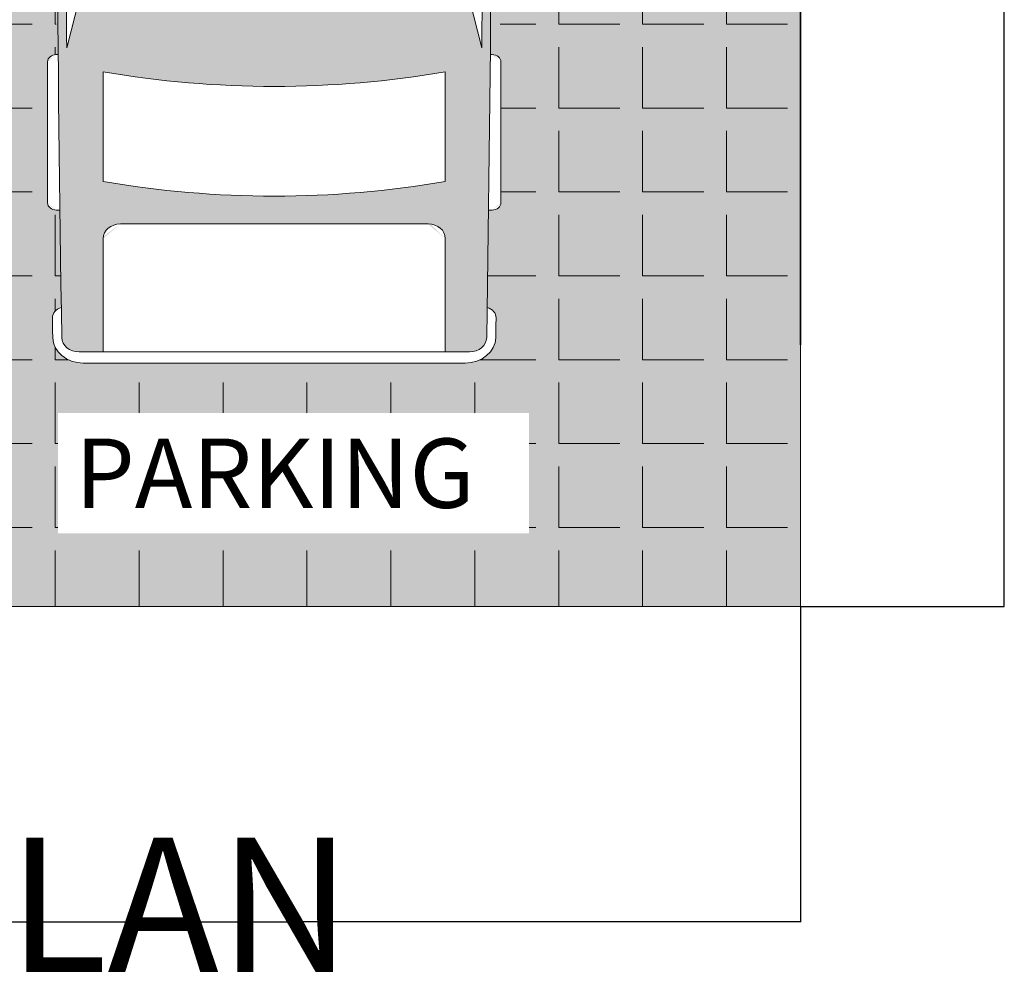
# Model space of a CAD drawing. Units: millimetres. Extents: x 1166 to 16630, y -7192 to 2820.
# Tile 4 of 8: x 5842 to 8218, y -7192 to -4887. Entities that reach past the tile are written whole.
import ezdxf

# ---------------------------------------------------------------- set-up
doc = ezdxf.new("R2010")
doc.units = ezdxf.units.MM
for name, color, linetype, lineweight in [('A-ANNO-DIMS', 2, 'Continuous', 18), ('A-ANNO-TEXT', 7, 'Continuous', 35), ('A-AREA-IDEN', 7, 'Continuous', 18), ('A-FLOR-PATT', 8, 'Continuous', 13), ('A-WALL', 7, 'Continuous', 35), ('C-PKNG-VEHI', 8, 'Continuous', 18), ('C-SITE-PAVE', 7, 'Continuous', 18)]:
    doc.layers.add(name, color=color, linetype=linetype, lineweight=lineweight)
doc.layers.add('A-FLOR-FNSH-PATT', color=254, linetype='Continuous', lineweight=13, true_color=0xfeeab9)
doc.layers.add('C-PKNG-VEHI-PATT', color=18, linetype='Continuous', lineweight=13, true_color=0x000000)
doc.styles.get("Standard").update_dxf_attribs({"font": 'arial.ttf'})
doc.dimstyles.get("Standard").update_dxf_attribs({"dimtxt": 0.18, "dimasz": 0.18, "dimexe": 0.18, "dimexo": 0.0625, "dimgap": 0.09, "dimtad": 0, "dimtih": 1, "dimtoh": 1, "dimdec": 4, "dimzin": 0, "dimdsep": 46, "dimtxsty": 'Standard', "dimcen": 0.09, "dimadec": 0, "dimazin": 0, "dimtfac": 1, "dimtdec": 4, "dimtofl": 0, "dimtmove": 0, "dimatfit": 3, "dimfxl": 1, "dimtolj": 1, "dimtzin": 0, "dimarcsym": 0})

# ---------------------------------------------------------------- blocks, each defined once
blk = doc.blocks.new('*U6')
for p, q in [((46.55368679439944, 38.88847654282876), (22.35054758993934, 38.88847654282876)), ((136.6978032355602, 38.88847654282876), (160.90094244002, 38.88847654282867)), ((21.10406751471477, 37.40863046792069), (21.10406751471477, 36.83230215753705)), ((47.80016686962392, 37.39011648242055), (47.80016686962392, 37.40863046792069)), ((135.4513231603356, 37.07354110333037), (135.4513231603356, 37.40863046792069)), ((162.1474225152445, 37.40863046792049), (162.1474225152445, 36.77402019194128)), ((87.98532186932616, 31.87120872459877), (74.75900729854769, 35.92175679182955)), ((134.313356548143, 35.6043097713567), (119.2882629232503, 31.77757799177584)), ((186.4728846989705, -33.49860931502491), (186.4728846989718, 33.49860931502465)), ((188.3990091454065, -32.75868627757393), (188.3990091454077, 32.75868627757058)), ((70.0302824853563, 31.53613089391356), (86.40615155322342, 29.35124891408057)), ((138.4228833961707, 29.35124891408074), (157.2465674415997, 29.35124891408074)), ((186.4728846989718, 29.35124891408083), (167.0083537481071, 29.35124891408083)), ((164.515393597658, 26.39155676426461), (164.5153935976578, -26.39155676426503)), ((32.26591480791686, 11.62530558863241), (36.12873726252356, 17.16961494239206)), ((36.12873726252356, 17.16961494239206), (50.93891189819171, 17.16961494239206)), ((32.12291633764599, 9.505833383620029), (32.12291633764599, 11.15369945057711)), ((58.9167604809788, -10.77488335095668), (58.9167604809788, 10.77488335095617)), ((66.55009204259746, -10.5288681329018), (66.55009204259746, 10.52886813290129)), ((186.4728846989718, -10.5288681329018), (186.4728846989718, 10.52886813290129)), ((29.77279020470884, 9.505833383620029), (51.68362801571248, 9.505833383620029)), ((82.73706193978568, 8.496039918672748), (82.73706193978568, -8.49603991867258)), ((3.266462181856987, 6.128290093440767), (0.1022408397004821, 0.4060708604429806)), ((-4.43e-14, -2.558e-13), (51.68362801571248, -2.558e-13)), ((0.1022408397004821, -0.4060708604432933), (3.266462181856987, -6.128290093441194)), ((29.77279020470884, -9.50583338362054), (51.68362801571248, -9.50583338362054)), ((32.12291633764599, -9.50583338362054), (32.12291633764599, -11.15369945057762)), ((32.26591480791686, -11.62530558863292), (36.12873726252356, -17.16961494239257)), ((36.12873726252356, -17.16961494239257), (50.93891189819171, -17.16961494239257)), ((86.40615155322318, -29.35124891408145), (70.03028248535594, -31.53613089391442)), ((157.2465674415997, -29.35124891408117), (138.4228833961707, -29.35124891408126)), ((167.008353748107, -29.35124891408126), (186.4728846989707, -29.35124891408108)), ((87.98532186932607, -31.87120872459903), (74.7590072985476, -35.92175679182964)), ((134.3133565481428, -35.60430977135721), (119.2882629232503, -31.77757799177618)), ((21.10406751471477, -37.4086304679212), (21.10406751471477, -36.83230215753756)), ((135.4513231603355, -37.07354110333088), (135.4513231603355, -37.4086304679212)), ((162.1474225152445, -37.408630467921), (162.1474225152445, -36.77402019194179)), ((47.80016686962392, -37.39011648242107), (47.80016686962392, -37.4086304679212)), ((46.55368679439944, -38.88847654282927), (22.35054758993934, -38.88847654282927)), ((136.6978032355602, -38.88847654282927), (160.9009424400199, -38.88847654282918))]:
    blk.add_line(p, q)
for centre, major_axis, ratio, start_param, end_param in [((22.35054758993934, 37.40863046792072), (2.08e-14, -1.479846074908118), 0.842303869543976, 3.141592653589776, 4.712388980384677), ((46.55368679439944, 37.40863046792072), (2.2e-14, 1.479846074908118), 0.8423038695439758, -1.570796326794884, 1.73e-14), ((136.6978032355602, 37.40863046792072), (2.357e-13, -1.479846074908118), 0.842303869543976, 3.141592653589603, 4.712388980384554), ((160.90094244002, 37.40863046792052), (5.59e-14, 1.479846074908118), 0.842303869543976, -1.570796326794865, 4.44e-14), ((41.19115208863305, -490.8631038926156), (1.294e-13, 528.2339998381949), 0.8423038695439741, 0.0028100083536837, 0.0755983031096952), ((64.48199294511879, -10555.61767587835), (1.907644e-10, 10593.02630634627), 0.842303869543847, -0.0133969486112073, 0.0027970409639888), ((180.6280394947615, 35.8381667808375), (7.4e-14, 2.219769112362114), 0.8423038695439693, -0.0130174256259048, 1.249894140392862), ((64.48199294754608, -10556.35759891604), (1.349839377e-06, 10595.3130398087), 0.8423038681351469, -0.0133969484821159, -0.0130174254969711), ((183.9799245485216, 32.75868627756583), (8.56e-14, -5.246425615115243), 0.8423038695439737, 1.570796326795794, 3.128195704978164), ((266.0300214172791, -27.52442688366631), (1.966072e-10, 313.3077612809058), 0.8423038695435284, 1.367075990158062, 1.391760499156098), ((64.4819929449925, -10555.61767590795), (1.9177683e-09, -10591.54646030096), 0.8423038695482963, 3.133765086725325, 3.140440689641252), ((183.9799245485226, 33.49860931502124), (3e-16, -2.959692149816168), 0.8423038695439952, 1.570796326796048, 3.128195704978389), ((135.2911776514449, 5.387441675478555), (2.2715e-12, 81.77258453065997), 0.8423038695439563, 1.245306111696802, 1.507880129813836), ((95.78879860270445, -3666.353346297651), (1.949864e-10, -3698.236159209632), 0.8423038695446962, 3.134048706297306, 3.14409775411291), ((37.47375371777758, -593.9621830607928), (6.21e-14, -623.32820996736), 0.8423038695439826, 3.09604606856106, 3.200911180495224), ((149.595361812917, 2.799442537139299), (8.561e-13, -79.57966406425402), 0.842303869543983, 4.372215489277867, 4.640744122441986), ((17.08207736189386, -1.421e-13), (6.87e-14, 147.0179238898305), 0.8423038695439764, 4.511394369635731, 4.913383591133647), ((35.90576140732288, -1.421e-13), (6.87e-14, 147.0179238898305), 0.8423038695439764, 4.511394369635731, 4.913383591133647), ((167.0083537481071, 26.39155676426464), (1.394e-13, 2.959692149816236), 0.842303869543976, 5.55e-14, 1.57079632679492), ((259.1750197310735, -27.52442688366614), (1.506617e-10, -305.3028914627677), 0.8423038695443789, 4.528606069860317, 4.561837674556238), ((134.4003789125686, 5.387441675477674), (4.276e-13, -89.7774543484738), 0.84230386954398, 4.44948196380473, 4.652344057257214), ((-204.4946649195746, 52.39684969293512), (4.12053e-11, -250.9602162198571), 0.8423038695441164, 1.385369446298923, 1.434372047871027), ((13.03653510440275, 17.00972444508943), (1.2303e-12, 27.41599049210566), 0.8423038695439277, 4.435146050259648, 4.718221029521873), ((14.20086229321332, 17.00972444508943), (1.2303e-12, 27.41599049210566), 0.8423038695439277, 4.435146050259648, 4.718221029521873), ((50.7902773840875, 13.33772416300607), (6.340077547122382, -0.356608581037027), 0.6038335755719145, -1.39555193967809, 1.581314658479915), ((32.74615637525823, 11.15369945057713), (1.313e-13, 0.7399230374541176), 0.8423038695439091, 0.8797135699495516, 1.570796326795045), ((29.77279020470884, -46.66302566589627), (5.12e-14, 56.16885904951626), 0.842303869543976, 7e-16, 0.5903187773915901), ((0.6232400376122422, -1.421e-13), (1e-16, -0.7399230374541245), 0.842303869543842, 4.131459131953847, 5.293318828815531), ((29.77279020470884, 46.66302566589578), (4.004e-13, 56.16885904951626), 0.8423038695439734, 2.55127387619821, 3.141592653589801), ((-204.4946649195746, -52.39684969293552), (4.02945e-11, 250.9602162198562), 0.8423038695441192, -1.43437204787103, -1.385369446298926), ((13.03653510440275, -17.00972444508983), (1.2568e-12, -27.41599049210552), 0.8423038695439318, 1.564964277657711, 1.848039256919935), ((14.20086229321332, -17.00972444508983), (1.2568e-12, -27.41599049210552), 0.8423038695439318, 1.564964277657711, 1.848039256919935), ((149.5953618129329, -2.799442537137565), (4.0897e-12, -79.57966406427697), 0.8423038695439419, -1.499151468852248, -1.230622835688196), ((32.74615637525823, -11.1536994505777), (1.3e-13, -0.7399230374541176), 0.8423038695439093, 4.712388980384541, 5.403471737230034), ((134.4003789125684, -5.387441675478584), (4.2949e-12, -89.77745434847827), 0.8423038695439354, -1.510751403667474, -1.307889310215002), ((135.2911776514465, -5.387441675480715), (3.2038e-12, -81.77258453066244), 0.8423038695439492, -1.50788012981387, -1.245306111696839), ((259.1750197310694, 27.52442688365929), (1.08535e-11, 305.3028914629043), 0.8423038695439974, 1.721347632622872, 1.754579237318777), ((167.008353748107, -26.39155676426503), (1.02e-14, -2.959692149816192), 0.8423038695439885, 4.712388980384686, 6.283185307179581), ((266.0300214172791, 27.52442688366566), (8.75241e-11, 313.3077612806533), 0.8423038695441819, 1.749832154434603, 1.774516663432659), ((37.47375371777847, 593.9621830607904), (1.1693e-12, -623.3282099673584), 0.8423038695439528, -0.0593185269054384, 0.0455465850287298), ((95.78879860271888, 3666.35334629765), (1.637818e-10, -3698.236159209629), 0.8423038695447546, -0.0025051005232382, 0.007543947292366), ((183.9799245485216, -33.4986093150211), (9.3e-15, 2.959692149816141), 0.8423038695439732, 3.154989602201626, 4.71238898038339), ((183.9799245485177, -32.7586862775633), (2.428e-13, -5.246425615118353), 0.8423038695439808, 0.0133969486110846, 1.570796326792831), ((41.19115208863322, 490.8631038926152), (1.37757e-11, -528.2339998381949), 0.8423038695440652, -0.0755983031097181, -0.0028100083537155), ((64.48199294495228, 10555.61767590795), (6.117947e-10, 10593.02630637587), 0.8423038695458146, 3.138795612625926, 3.154989602201039), ((64.48199294503607, 10555.61767590793), (1.6049794e-09, -10591.54646030094), 0.8423038695397146, 0.0011519639481523, 0.0078275668641468), ((180.6280394947581, -35.83816678083949), (2.274e-13, -2.219769112363032), 0.8423038695439803, -1.249894138785958, 0.0130174256254374), ((22.35054758993934, -37.40863046792117), (2.2e-14, 1.479846074908118), 0.8423038695439758, 1.570796326794908, 3.14159265358981), ((46.55368679439944, -37.40863046792117), (2.08e-14, -1.479846074908118), 0.842303869543976, -1.69e-14, 1.570796326794884), ((136.6978032355602, -37.40863046792109), (1.56e-14, -1.479846074908162), 0.8423038695440105, -1.570796326794875, -1.27e-14), ((160.9009424400199, -37.408630467921), (1.969e-13, 1.479846074908162), 0.8423038695440109, 3.141592653589951, 4.712388980384771), ((64.48199294197605, 10556.3575989598), (9.365289701e-07, 10595.31303985772), 0.8423038705260315, 3.154610079306566, 3.154989602290631)]:
    blk.add_ellipse(centre, major_axis=major_axis, ratio=ratio, start_param=start_param, end_param=end_param)
at = {"extrusion": (0, 0, -1)}
blk.add_ellipse((50.7902773840875, -13.33772416300655), major_axis=(6.340077547122382, 0.3566085810370246), ratio=0.6038335755719145, start_param=-1.39555193967809, end_param=1.581314658479915, dxfattribs=at)
blk = doc.blocks.new('*D24')
at = {"layer": 'A-ANNO-DIMS', "color": 0, "lineweight": -2, "transparency": 16777216}
for p, q in [((7726.001941000004, 2327.462235000001), (8218.11944100001, 2327.462235000001)), ((8217.93944100001, 2327.282235000001), (8217.93944100001, -1988.15746197067)), ((8217.939441000011, -6303.961088000004), (8217.93944100001, -1988.521391029333)), ((7726.001941000004, -6304.141088000005), (8218.119441000012, -6304.141088000005))]:
    blk.add_line(p, q, dxfattribs=at)
at = {"layer": 'A-ANNO-DIMS', "color": 0, "transparency": 16777216}
for points in [[(8217.909441000009, 2327.282235000001), (8217.969441000008, 2327.282235000001), (8217.93944100001, 2327.462235000001)], [(8217.909441000009, -6303.961088000004), (8217.96944100001, -6303.961088000004), (8217.939441000011, -6304.141088000005)]]:
    blk.add_solid(points, dxfattribs=at)
at = {"layer": 'Defpoints', "color": 0, "transparency": 16777216}
for p in [(7725.939441000004, 2327.462235000001), (7725.939441000004, -6304.141088000005), (8217.939441000011, -6304.141088000005)]:
    blk.add_point(p, dxfattribs=at)
at = {"layer": 'A-ANNO-DIMS', "color": 0, "transparency": 16777216, "insert": (8217.939441000006, -1988.339426500003), "char_height": 0.18, "attachment_point": 5}
blk.add_mtext('\\A1;8632', dxfattribs=at)
blk = doc.blocks.new('*D32')
at = {"layer": 'A-ANNO-DIMS', "color": 0, "lineweight": -2, "transparency": 16777216}
for p, q in [((5309.614993, -6304.203588), (5309.614993, -7065.629165)), ((7725.939441000001, -6304.203588), (7725.939441000001, -7065.629165)), ((5309.794993, -7065.449165), (6517.312053289224, -7065.449165)), ((7725.759441000001, -7065.449165), (6518.242380710778, -7065.449165))]:
    blk.add_line(p, q, dxfattribs=at)
at = {"layer": 'A-ANNO-DIMS', "color": 0, "transparency": 16777216}
for points in [[(5309.794993, -7065.419165), (5309.794993, -7065.479164999999), (5309.614993, -7065.449165)], [(7725.759441000001, -7065.419165), (7725.759441000001, -7065.479164999999), (7725.939441000001, -7065.449165)]]:
    blk.add_solid(points, dxfattribs=at)
at = {"layer": 'Defpoints', "color": 0, "transparency": 16777216}
for p in [(5309.614993, -6304.141088000001), (7725.939441000001, -6304.141088000001), (7725.939441000001, -7065.449165)]:
    blk.add_point(p, dxfattribs=at)
at = {"layer": 'A-ANNO-DIMS', "color": 0, "transparency": 16777216, "insert": (6517.777217000001, -7065.449165), "char_height": 0.18, "attachment_point": 5}
blk.add_mtext('\\A1;2416.3', dxfattribs=at)

msp = doc.modelspace()

# ---------------------------------------------------------------- hatches: boundary and pattern name
at = {"layer": 'A-FLOR-FNSH-PATT', "transparency": 33554590}
h = msp.add_hatch(color=256, dxfattribs=at)
h.dxf.hatch_style = 1
h.paths.add_polyline_path([(5309.614992693758, -2642.53776490782), (5309.614992693758, -6304.141088113749), (7725.939441137629, -6304.141088113749), (7725.939441137629, -5672.53776490782), (7725.939441137629, -2642.53776490782)])
edge = h.paths.add_edge_path(flags=16)
edge.add_ellipse((-448.9724108440159, -3645.429588524165), major_axis=(-7430.722679011307, 2.05049e-10), ratio=0.8423038695440578, start_angle=182.1799503136468, end_angle=183.6504275857006, ccw=False)
edge.add_line((6974.17381326888, -3362.862478220109), (6984.715647929133, -3362.862478220109))
edge.add_ellipse((6982.28108362224, -3380.396843230207), major_axis=(-20.81714882728829, 5.19e-13), ratio=0.842303869543992, start_angle=180.0000000000014, end_angle=270.0000000000014, ccw=False)
edge.add_line((7003.098232449528, -3380.396843230198), (7003.098232449528, -3722.915565549822))
edge.add_ellipse((6982.28108362224, -3720.864922613471), major_axis=(20.81714882728829, 5.097e-13), ratio=0.842303869543992, start_angle=269.9999999999985, end_angle=359.9999999999986, ccw=False)
edge.add_ellipse((-142030.922985108, -3973.064272051784), major_axis=(149013.2040687302, 7.3876543e-09), ratio=0.8423038695454406, start_angle=-0.3838667787953227, end_angle=0.09022908859151357, ccw=False)
edge.add_line((6977.567346638728, -4971.397229994678), (6984.470063297348, -4971.397229994678))
edge.add_ellipse((6982.28108362224, -4988.931595004776), major_axis=(20.81714882728829, 5.4695e-12), ratio=0.84230386954397, start_angle=-1.5006662579253316e-11, end_angle=89.99999999998488, ccw=False)
edge.add_line((7003.098232449528, -4988.931595004766), (7003.098232449527, -5331.243460438734))
edge.add_ellipse((6982.281083622239, -5329.399674388036), major_axis=(-20.81714882728829, 1.0505e-12), ratio=0.84230386954397, start_angle=90.0000000000029, end_angle=180.000000000003, ccw=False)
edge.add_line((6982.281083622243, -5346.934039398132), (6973.353954790083, -5346.934039398132))
edge.add_ellipse((-142030.922985108, -3973.064272051784), major_axis=(149013.2040687302, 7.3876543e-09), ratio=0.8423038695454406, start_angle=-0.6186431963221253, end_angle=-0.5282714718208013, ccw=False)
edge.add_ellipse((6960.189207408767, -5606.902802775503), major_axis=(-31.22572324093233, 2.0889e-12), ratio=0.8423038695439425, start_angle=179.3717627838109, end_angle=248.4647566010108, ccw=False)
edge.add_ellipse((-142041.331559525, -3973.064272085929), major_axis=(-149045.3717863939, 4.64621177404e-05), ratio=0.8423038661083152, start_angle=179.3534459208122, end_angle=179.3717628016453, ccw=False)
edge.add_ellipse((6916.869834512962, -5654.054118847628), major_axis=(-73.80201542105252, 3.6097e-12), ratio=0.8423038695439748, start_angle=90.00000000006492, end_angle=179.353445902922, ccw=False)
edge.add_line((6916.869834513031, -5716.217842016925), (5995.230132669023, -5716.217842016909))
edge.add_ellipse((5995.230132669163, -5654.054118847574), major_axis=(73.80201542109666, 3.978e-13), ratio=0.8423038695439887, start_angle=180.6465540970575, end_angle=269.9999999998622, ccw=False)
edge.add_ellipse((154953.4315273228, -3973.06427200764), major_axis=(-149045.3717871212, 2.2898328512e-06), ratio=0.8423038697262194, start_angle=0.6282372171232851, end_angle=0.6465540979564253, ccw=False)
edge.add_ellipse((5951.910759773294, -5606.902802775455), major_axis=(31.22572324094488, 4.9039e-12), ratio=0.842303869543988, start_angle=111.53524350401449, end_angle=180.6282372161637, ccw=False)
edge.add_ellipse((154943.0229527065, -3973.064272049507), major_axis=(-149013.2040691466, 7.4869171e-09), ratio=0.8423038695459824, start_angle=0.528271471820176, end_angle=0.6465540970638131, ccw=False)
edge.add_line((5938.746012391977, -5346.934039398132), (5927.384319252956, -5346.934039398132))
edge.add_ellipse((5929.818883559845, -5329.399674388033), major_axis=(20.8171488272892, 3.11e-13), ratio=0.8423038695440205, start_angle=179.9999999999992, end_angle=269.9999999999962, ccw=False)
edge.add_line((5909.001734732555, -5329.399674388034), (5909.001734732554, -4986.88095206843))
edge.add_ellipse((5929.818883559843, -4988.931595004776), major_axis=(-20.8171488272892, 3.063e-13), ratio=0.8423038695440205, start_angle=-89.99999999999608, end_angle=7.958078640513122e-13, ccw=False)
edge.add_line((5929.818883559843, -4971.397229994676), (5934.53262054336, -4971.397229994676))
edge.add_ellipse((154943.0229527065, -3973.064272049507), major_axis=(-149013.2040691466, 7.4869171e-09), ratio=0.8423038695459824, start_angle=-0.09022908859031986, end_angle=0.38386677879520903, ccw=False)
edge.add_ellipse((5929.818883559843, -3720.864922613471), major_axis=(-20.8171488272892, 1.5867e-12), ratio=0.8423038695439331, start_angle=4.376943252282217e-12, end_angle=90.00000000000438, ccw=False)
edge.add_line((5909.001734732555, -3720.864922613478), (5909.001734732555, -3378.346200293855))
edge.add_ellipse((5929.818883559843, -3380.396843230207), major_axis=(20.8171488272892, 9.396e-13), ratio=0.8423038695439548, start_angle=89.99999999999739, end_angle=179.9999999999975, ccw=False)
edge.add_line((5929.818883559843, -3362.862478220109), (5937.926153913206, -3362.862478220109))
edge.add_ellipse((13361.0723780261, -3645.42958852417), major_axis=(7430.722679011307, 7.96527e-11), ratio=0.8423038695440075, start_angle=176.3495724143003, end_angle=177.8200496863542, ccw=False)
edge.add_ellipse((6843.238962592569, -6808.26137511002), major_axis=(4407.332901654202, 4.993684e-10), ratio=0.8423038695438785, start_angle=102.12596555227748, end_angle=103.7805289894913, ccw=False)
edge.add_ellipse((6843.238962592481, -6711.831352601092), major_axis=(4294.727564406183, 8.108409e-10), ratio=0.8423038695438188, start_angle=100.20953899713243, end_angle=102.4446272934332, ccw=False)
edge.add_ellipse((5718.978043047074, -189.3416182050969), major_axis=(-3530.283493235897, 2.29487e-11), ratio=0.8423038695439934, start_angle=99.25656600720184, end_angle=102.5549326441376)
edge.add_line((6369.842688727707, -3111.939026631001), (6452.046781461999, -3066.482546539763))
edge.add_ellipse((6456.049983591043, -3074.756545497792), major_axis=(-10.40857441364578, 1.5838e-12), ratio=0.8423038695437935, start_angle=270.0000000000206, end_angle=307.9331304598557, ccw=False)
edge.add_ellipse((6456.049983591043, -3074.756545497792), major_axis=(-10.40857441364578, 1.5838e-12), ratio=0.8423038695437935, start_angle=232.06686954016618, end_angle=270.0000000000206, ccw=False)
edge.add_line((6461.762224667734, -3067.427595530816), (6542.257278454378, -3111.939026631002))
edge.add_ellipse((7193.121924135012, -189.3416182050969), major_axis=(3530.283493235459, 5.426614e-10), ratio=0.842303869544094, start_angle=257.4450673558539, end_angle=260.7434339927895)
edge.add_ellipse((6068.861004589511, -6711.831352601148), major_axis=(4294.72756440461, 7.517164e-10), ratio=0.8423038695441345, start_angle=77.55537270654469, end_angle=79.79046100284552, ccw=False)
edge.add_ellipse((6068.86100458951, -6808.26137511002), major_axis=(-4407.332901654327, 6.637773e-10), ratio=0.842303869543856, start_angle=256.2194710105107, end_angle=257.8740344477245, ccw=False)
edge = h.paths.add_edge_path(flags=0)
edge.add_ellipse((5799.636342679871, -3484.80630294614), major_axis=(790.1331889300527, 2.1537e-12), ratio=0.8423038695439757, start_angle=-2.2737367544323206e-13, end_angle=29.43856959797921, ccw=False)
edge.add_line((6589.769531609924, -3484.806302946152), (6589.769531609924, -3517.865771969153))
edge.add_line((6589.769531609924, -3517.865771969153), (6615.396946753699, -3517.865771969153))
edge.add_ellipse((6612.950235160742, -3526.632954474201), major_axis=(10.40857441364348, 1.5653e-12), ratio=0.8423038695440233, start_angle=45.51978911742219, end_angle=89.99999999999147, ccw=False)
edge.add_line((6619.58436781158, -3519.877346340421), (6697.576744801804, -3574.216072032502))
edge.add_line((6697.576744801804, -3574.216072032502), (6697.576744801804, -3782.552340767745))
edge.add_ellipse((6643.673138205864, -3780.461483581003), major_axis=(5.016450041930374, 89.18653102701357), ratio=0.6038335755719256, start_angle=106.34259195429391, end_angle=270.99798572497, ccw=False)
edge.add_line((6589.769531609924, -3793.028339937766), (6589.769531609924, -3484.806302946153))
edge.add_ellipse((5799.636342679871, -3484.80630294614), major_axis=(790.1331889300527, 2.1537e-12), ratio=0.8423038695439757, start_angle=-2.143e-13, end_angle=29.43856959797918)
edge.add_ellipse((7112.463624502211, -3484.80630294614), major_axis=(-790.1331889300524, 7.9434e-12), ratio=0.8423038695439707, start_angle=-29.43856959797882, end_angle=5.465e-13)
edge.add_line((6322.330435572158, -3484.806302946151), (6322.330435572158, -3793.028339937766))
edge.add_ellipse((6268.426828976219, -3780.461483581003), major_axis=(-5.016450041930374, 89.18653102701357), ratio=0.6038335755719256, start_angle=89.00201427502998, end_angle=253.6574080457062, ccw=False)
edge.add_line((6214.523222380278, -3782.552340767737), (6214.523222380279, -3574.216072032502))
edge.add_line((6214.523222380279, -3574.216072032502), (6294.400928520307, -3518.563802793423))
edge.add_ellipse((6299.149732021341, -3526.632954474201), major_axis=(10.4085744136453, 3.381e-13), ratio=0.8423038695438764, start_angle=89.9999999999983, end_angle=134.4802108825654, ccw=False)
edge.add_line((6299.149732021338, -3517.865771969152), (6322.330435572158, -3517.865771969152))
edge.add_line((6322.330435572158, -3517.865771969152), (6322.330435572158, -3484.806302946154))
edge.add_ellipse((7112.463624502211, -3484.80630294614), major_axis=(-790.1331889300524, 7.9434e-12), ratio=0.8423038695439707, start_angle=-29.438569597978812, end_angle=6.252776074688882e-13, ccw=False)
edge = h.paths.add_edge_path(flags=0)
edge.add_line((6899.672020630411, -4051.112638739672), (6868.937058315451, -4281.473694083312))
edge.add_ellipse((6495.430033257824, -5170.362894493258), major_axis=(1119.455420763322, 3.0514e-12), ratio=0.8423038695439744, start_angle=67.20808512240981, end_angle=85.12993040286408)
edge.add_line((6575.564661792019, -4229.860228440724), (6336.53530539007, -4229.860228440724))
edge.add_ellipse((6416.669933924288, -5170.362894493482), major_axis=(1119.455420763633, 5.82337e-11), ratio=0.842303869543943, start_angle=94.87006959713275, end_angle=112.7919148775836)
edge.add_line((6043.162908866626, -4281.473694083309), (6012.427946551666, -4051.112638739666))
edge.add_ellipse((6380.264280565288, -4969.144446445703), major_axis=(1150.303461305961, 5.9583e-11), ratio=0.8423038695439412, start_angle=94.27742096305099, end_angle=111.83495379670521, ccw=False)
edge.add_line((6307.939299228742, -4002.156437400477), (6604.160667953341, -4002.156437400477))
edge.add_ellipse((6531.835686616772, -4969.144446445682), major_axis=(-1150.303461305901, 2.25473e-11), ratio=0.8423038695439672, start_angle=248.1650462032914, end_angle=265.72257903694555, ccw=False)
edge = h.paths.add_edge_path(flags=0)
edge.add_ellipse((-142030.9229855244, -3973.064272050007), major_axis=(-148992.3869203194, 2.076209e-10), ratio=0.842303869544003, start_angle=179.6222358060902, end_angle=179.9444056865007, ccw=False)
edge.add_line((6956.899516505626, -4955.389335168179), (6903.06848209712, -4744.029778632651))
edge.add_ellipse((-45118.92430422086, -4413.460367112857), major_axis=(52023.47313689829, 7.771381e-10), ratio=0.842303869543516, start_angle=-0.3640763488911976, end_angle=0.1208973690317991)
edge.add_line((6904.3855953652, -4303.688047353878), (6961.365076797346, -4117.63210307358))
edge = h.paths.add_edge_path(flags=0)
edge.add_line((5950.734890384741, -4117.632103073563), (6007.714371816899, -4303.688047353918))
edge.add_ellipse((58031.02427140294, -4413.460367113082), major_axis=(-52023.47313689826, 1.3200601e-09), ratio=0.8423038695497072, start_angle=-0.1208973690315197, end_angle=0.364076348891516)
edge.add_line((6009.031485084967, -4744.029778632643), (5955.200450676423, -4955.389335168309))
edge.add_ellipse((154943.0229527063, -3973.064272050686), major_axis=(-148992.3869203192, 3.28274152e-08), ratio=0.8423038695536886, start_angle=0.05559431351167632, end_angle=0.3777641939223031, ccw=False)
edge = h.paths.add_edge_path(flags=0)
edge.add_line((6868.937058315452, -5013.198477251068), (6868.937058315452, -5277.993200767081))
edge.add_ellipse((6456.049983591043, -3571.079447459644), major_axis=(2068.11644385622, 7.9333e-12), ratio=0.8423038695439821, start_angle=256.4018653097692, end_angle=283.59813469023027, ccw=False)
edge.add_line((6043.16290886663, -5277.993200767081), (6043.16290886663, -5013.198477251068))
edge.add_ellipse((6456.049983591043, -3306.284723943631), major_axis=(2068.116443856253, 3.3411e-12), ratio=0.8423038695439679, start_angle=256.4018653097692, end_angle=283.5981346902304)
edge = h.paths.add_edge_path(flags=0)
edge.add_ellipse((6827.302760660877, -5415.313265203762), major_axis=(-41.63429765457658, 1.038e-12), ratio=0.842303869543992, start_angle=180.0000000000014, end_angle=270.0000000000014, ccw=False)
edge.add_line((6868.937058315454, -5415.313265203762), (6868.937058315454, -5689.12284886784))
edge.add_line((6868.937058315454, -5689.12284886784), (6043.162908866631, -5689.122848867824))
edge.add_line((6043.162908866631, -5689.122848867824), (6043.16290886663, -5415.313265203758))
edge.add_ellipse((6084.797206521206, -5415.313265203759), major_axis=(-41.63429765457658, 3.4138e-12), ratio=0.842303869543992, start_angle=-89.99999999999523, end_angle=4.718003765447065e-12, ccw=False)
edge.add_line((6084.797206521207, -5380.244535183563), (6827.302760660879, -5380.244535183566))
h.paths.add_polyline_path([(3455.939441137629, -522.53776490782), (1955.939441137629, -522.53776490782), (1955.939441137629, -2522.53776490782), (3455.939441137629, -2522.53776490782), (3455.939441137628, -2456.640093510054), (2713.439441137629, -2456.640093510054), (2713.43944113763, -2423.827593510054), (2714.157558370035, -2423.827593510054, -0.398552660000795), (3455.939441137629, -1706.6775944476)])
h.paths.add_polyline_path([(2617.666699633915, -1084.404517764245, -0.1328909081885223), (2584.2707950462, -1084.404517500826, -0.5013167773008519), (2505.064916213601, -782.9330743979599), (2537.033121160981, -687.0284595558127), (2489.081652205778, -687.0284595558132), (2489.081652205778, -711.0041940334158), (2441.130183250573, -711.0041940334158), (2441.130183250573, -695.0203710483474), (2473.097829220709, -695.0203710483474), (2473.097829220709, -687.0284595558132), (2433.13827175804, -687.0284595558132), (2433.138271758038, -559.1578756752674), (2768.79855444447, -559.1578756752674), (2768.798554444471, -687.0284595558132), (2664.903705041528, -687.0284595558132), (2696.870765296628, -782.9296403211174, -0.5013234908365807)], flags=16)
h.paths.add_polyline_path([(2627.246667254758, -1063.015793855155, -0.2150037826753064), (2574.690827957319, -1063.015793301825, -0.4800796505537303), (2537.033991046725, -782.9313974662227), (2664.904416594217, -782.9313974662227, -0.4800795019660876)], flags=0)
h.paths.add_polyline_path([(2736.830905816404, -671.0446365707452), (2465.105920386107, -671.0446365707452, -0.5000001164022092), (2449.122094743107, -655.0608109277463), (2449.122094743107, -591.1255243033341, -0.5000001164022404), (2465.105920386111, -575.1416986603361), (2736.830905816402, -575.1416986603361, -0.5000001164023353), (2752.814731459403, -591.1255243033406), (2752.814731459403, -655.0608109277468, -0.50000011640211)], flags=0)
h.paths.add_polyline_path([(5931.781743219382, -6111.826019846759), (7070.309755611069, -6111.826019846759), (7070.309755611069, -5852.301891921869), (5931.781743219382, -5852.301891921869)], flags=24)
h.paths.add_polyline_path([(2102.335631979146, -1543.656328414819), (3007.075088498303, -1543.656328414819), (3007.075088498303, -1283.961010431932), (2102.335631979146, -1283.961010431932)], flags=24)
at = {"layer": 'A-FLOR-PATT', "transparency": 33554564}
h = msp.add_hatch(dxfattribs=at)
h.set_pattern_fill('ANGLE', color=256, scale=29)
h.set_pattern_definition([(0, (-8657.519420588213, -11987.85165359825), (0, 202.565), [147.32, -55.24499999999999]), (90, (-8657.519420588213, -11987.85165359825), (-202.565, 1.24e-14), [147.32, -55.24499999999999])])
h.paths.add_polyline_path([(7725.939441137629, -2642.53776490782), (5309.614992693758, -2642.53776490782), (5309.614992693758, -6304.141088113749), (7725.939441137629, -6304.141088113749), (7725.939441137629, -5672.53776490782)])
edge = h.paths.add_edge_path(flags=16)
edge.add_ellipse((-142030.922985108, -3973.064272051784), major_axis=(149013.2040687302, 7.3876543e-09), ratio=0.8423038695454406, start_angle=-0.3838667787953227, end_angle=0.09022908859151357, ccw=False)
edge.add_ellipse((6982.28108362224, -4988.931595004776), major_axis=(20.81714882728829, 5.4695e-12), ratio=0.84230386954397, start_angle=-1.5006662579253316e-11, end_angle=89.99999999998488, ccw=False)
edge.add_line((7003.098232449528, -4988.931595004773), (7003.098232449527, -5329.399674388036))
edge.add_ellipse((6982.281083622239, -5329.399674388036), major_axis=(-20.81714882728829, 1.0505e-12), ratio=0.84230386954397, start_angle=90.0000000000029, end_angle=180.000000000003, ccw=False)
edge.add_line((6982.281083622241, -5346.934039398132), (6973.353954790083, -5346.934039398132))
edge.add_ellipse((-142030.922985108, -3973.064272051784), major_axis=(149013.2040687302, 7.3876543e-09), ratio=0.8423038695454406, start_angle=-0.6186431963221253, end_angle=-0.5282714718208013, ccw=False)
edge.add_ellipse((6960.189207408767, -5606.902802775503), major_axis=(-31.22572324093233, 2.0889e-12), ratio=0.8423038695439425, start_angle=179.3717627838109, end_angle=248.4647566010108, ccw=False)
edge.add_ellipse((-142041.331559525, -3973.064272085929), major_axis=(-149045.3717863939, 4.64621177404e-05), ratio=0.8423038661083152, start_angle=179.3534459208122, end_angle=179.3717628016453, ccw=False)
edge.add_ellipse((6916.869834512962, -5654.054118847628), major_axis=(-73.80201542105252, 3.6097e-12), ratio=0.8423038695439748, start_angle=90.00000000006492, end_angle=179.353445902922, ccw=False)
edge.add_line((6916.869834513029, -5716.217842016925), (5995.230132669016, -5716.217842016909))
edge.add_ellipse((5995.230132669163, -5654.054118847574), major_axis=(73.80201542109666, 3.978e-13), ratio=0.8423038695439887, start_angle=180.6465540970575, end_angle=269.9999999998622, ccw=False)
edge.add_ellipse((154953.4315273228, -3973.06427200764), major_axis=(-149045.3717871212, 2.2898328512e-06), ratio=0.8423038697262194, start_angle=0.6282372171232851, end_angle=0.6465540979564253, ccw=False)
edge.add_ellipse((5951.910759773294, -5606.902802775455), major_axis=(31.22572324094488, 4.9039e-12), ratio=0.842303869543988, start_angle=111.53524350401449, end_angle=180.6282372161637, ccw=False)
edge.add_ellipse((154943.0229527065, -3973.064272049507), major_axis=(-149013.2040691466, 7.4869171e-09), ratio=0.8423038695459824, start_angle=0.528271471820176, end_angle=0.6465540970638131, ccw=False)
edge.add_line((5938.746012391977, -5346.934039398132), (5929.818883559843, -5346.934039398132))
edge.add_ellipse((5929.818883559845, -5329.399674388033), major_axis=(20.8171488272892, 3.11e-13), ratio=0.8423038695440205, start_angle=179.9999999999992, end_angle=269.9999999999962, ccw=False)
edge.add_line((5909.001734732555, -5329.399674388033), (5909.001734732554, -4988.931595004778))
edge.add_ellipse((5929.818883559843, -4988.931595004776), major_axis=(-20.8171488272892, 3.063e-13), ratio=0.8423038695440205, start_angle=-89.99999999999608, end_angle=7.958078640513122e-13, ccw=False)
edge.add_ellipse((154943.0229527065, -3973.064272049507), major_axis=(-149013.2040691466, 7.4869171e-09), ratio=0.8423038695459824, start_angle=-0.09022908859031986, end_angle=0.38386677879520903, ccw=False)
edge.add_ellipse((5929.818883559843, -3720.864922613471), major_axis=(-20.8171488272892, 1.5867e-12), ratio=0.8423038695439331, start_angle=4.376943252282217e-12, end_angle=90.00000000000438, ccw=False)
edge.add_line((5909.001734732555, -3720.864922613472), (5909.001734732555, -3380.396843230204))
edge.add_ellipse((5929.818883559843, -3380.396843230207), major_axis=(20.8171488272892, 9.396e-13), ratio=0.8423038695439548, start_angle=89.99999999999739, end_angle=179.9999999999975, ccw=False)
edge.add_line((5929.818883559843, -3362.862478220109), (5937.926153913207, -3362.862478220109))
edge.add_ellipse((13361.0723780261, -3645.42958852417), major_axis=(7430.722679011307, 7.96527e-11), ratio=0.8423038695440075, start_angle=176.3495724143003, end_angle=177.8200496863542, ccw=False)
edge.add_ellipse((6843.238962592569, -6808.26137511002), major_axis=(4407.332901654202, 4.993684e-10), ratio=0.8423038695438785, start_angle=102.12596555227748, end_angle=103.7805289894913, ccw=False)
edge.add_ellipse((6843.238962592481, -6711.831352601092), major_axis=(4294.727564406183, 8.108409e-10), ratio=0.8423038695438188, start_angle=100.20953899713243, end_angle=102.4446272934332, ccw=False)
edge.add_ellipse((5718.978043047074, -189.3416182050969), major_axis=(-3530.283493235897, 2.29487e-11), ratio=0.8423038695439934, start_angle=99.25656600720184, end_angle=102.5549326441376)
edge.add_line((6369.842688727707, -3111.939026631), (6453.505541262713, -3065.675894661087))
edge.add_ellipse((6456.049983591043, -3074.756545497792), major_axis=(-10.40857441364578, 1.5838e-12), ratio=0.8423038695437935, start_angle=232.06686954016618, end_angle=270.0000000000206, ccw=False)
edge.add_line((6460.053185720086, -3066.482546539763), (6542.257278454378, -3111.939026631002))
edge.add_ellipse((7193.121924135012, -189.3416182050969), major_axis=(3530.283493235459, 5.426614e-10), ratio=0.842303869544094, start_angle=257.4450673558539, end_angle=260.7434339927895)
edge.add_ellipse((6068.861004589511, -6711.831352601148), major_axis=(4294.72756440461, 7.517164e-10), ratio=0.8423038695441345, start_angle=77.55537270654469, end_angle=79.79046100284552, ccw=False)
edge.add_ellipse((6068.86100458951, -6808.26137511002), major_axis=(-4407.332901654327, 6.637773e-10), ratio=0.842303869543856, start_angle=256.2194710105107, end_angle=257.8740344477245, ccw=False)
edge.add_ellipse((-448.9724108440159, -3645.429588524165), major_axis=(-7430.722679011307, 2.05049e-10), ratio=0.8423038695440578, start_angle=182.1799503136468, end_angle=183.6504275857006, ccw=False)
edge.add_line((6974.17381326888, -3362.862478220109), (6982.28108362224, -3362.862478220109))
edge.add_ellipse((6982.28108362224, -3380.396843230207), major_axis=(-20.81714882728829, 5.19e-13), ratio=0.842303869543992, start_angle=180.0000000000014, end_angle=270.0000000000014, ccw=False)
edge.add_line((7003.098232449528, -3380.396843230204), (7003.098232449528, -3720.864922613474))
edge.add_ellipse((6982.28108362224, -3720.864922613471), major_axis=(20.81714882728829, 5.097e-13), ratio=0.842303869543992, start_angle=269.9999999999985, end_angle=359.9999999999986, ccw=False)
edge = h.paths.add_edge_path(flags=0)
edge.add_ellipse((-142030.9229855244, -3973.064272050007), major_axis=(-148992.3869203194, 2.076209e-10), ratio=0.842303869544003, start_angle=179.6222358060902, end_angle=179.9444056865007, ccw=False)
edge.add_line((6956.899516505626, -4955.389335168179), (6903.06848209712, -4744.029778632651))
edge.add_ellipse((-45118.92430422086, -4413.460367112857), major_axis=(52023.47313689829, 7.771381e-10), ratio=0.842303869543516, start_angle=-0.3640763488911976, end_angle=0.1208973690317991)
edge.add_line((6904.3855953652, -4303.688047353878), (6961.365076797346, -4117.632103073563))
edge = h.paths.add_edge_path(flags=0)
edge.add_line((6899.672020630411, -4051.112638739673), (6868.937058315451, -4281.473694083312))
edge.add_ellipse((6495.430033257824, -5170.362894493258), major_axis=(1119.455420763322, 3.0514e-12), ratio=0.8423038695439744, start_angle=67.20808512240981, end_angle=85.12993040286408)
edge.add_line((6575.564661792022, -4229.860228440724), (6336.535305390071, -4229.860228440724))
edge.add_ellipse((6416.669933924288, -5170.362894493482), major_axis=(1119.455420763633, 5.82337e-11), ratio=0.842303869543943, start_angle=94.87006959713275, end_angle=112.7919148775836)
edge.add_line((6043.162908866626, -4281.473694083308), (6012.427946551666, -4051.112638739666))
edge.add_ellipse((6380.264280565288, -4969.144446445703), major_axis=(1150.303461305961, 5.9583e-11), ratio=0.8423038695439412, start_angle=94.27742096305099, end_angle=111.83495379670521, ccw=False)
edge.add_line((6307.939299228742, -4002.156437400477), (6604.16066795334, -4002.156437400477))
edge.add_ellipse((6531.835686616772, -4969.144446445682), major_axis=(-1150.303461305901, 2.25473e-11), ratio=0.8423038695439672, start_angle=248.1650462032914, end_angle=265.72257903694555, ccw=False)
edge = h.paths.add_edge_path(flags=0)
edge.add_ellipse((6643.673138205864, -3780.461483581003), major_axis=(5.016450041930374, 89.18653102701357), ratio=0.6038335755719256, start_angle=106.34259195429391, end_angle=270.99798572497, ccw=False)
edge.add_line((6589.769531609924, -3793.028339937766), (6589.769531609924, -3484.806302946154))
edge.add_ellipse((5799.636342679871, -3484.80630294614), major_axis=(790.1331889300527, 2.1537e-12), ratio=0.8423038695439757, start_angle=-2.143e-13, end_angle=29.43856959797918)
edge.add_ellipse((7112.463624502211, -3484.80630294614), major_axis=(-790.1331889300524, 7.9434e-12), ratio=0.8423038695439707, start_angle=-29.43856959797882, end_angle=5.465e-13)
edge.add_line((6322.330435572158, -3484.806302946151), (6322.330435572158, -3793.028339937766))
edge.add_ellipse((6268.426828976219, -3780.461483581003), major_axis=(-5.016450041930374, 89.18653102701357), ratio=0.6038335755719256, start_angle=89.00201427502998, end_angle=253.6574080457062, ccw=False)
edge.add_line((6214.523222380278, -3782.552340767735), (6214.523222380279, -3574.216072032502))
edge.add_line((6214.523222380279, -3574.216072032502), (6295.402812213822, -3517.865771969152))
edge.add_line((6295.402812213822, -3517.865771969152), (6322.330435572158, -3517.865771969152))
edge.add_line((6322.330435572158, -3517.865771969152), (6322.330435572158, -3484.806302946154))
edge.add_ellipse((7112.463624502211, -3484.80630294614), major_axis=(-790.1331889300524, 7.9434e-12), ratio=0.8423038695439707, start_angle=-29.438569597978812, end_angle=6.252776074688882e-13, ccw=False)
edge.add_ellipse((5799.636342679871, -3484.80630294614), major_axis=(790.1331889300527, 2.1537e-12), ratio=0.8423038695439757, start_angle=-2.2737367544323206e-13, end_angle=29.43856959797921, ccw=False)
edge.add_line((6589.769531609924, -3484.806302946153), (6589.769531609924, -3517.865771969153))
edge.add_line((6589.769531609924, -3517.865771969153), (6616.697154968261, -3517.865771969153))
edge.add_line((6616.697154968261, -3517.865771969153), (6697.576744801804, -3574.216072032502))
edge.add_line((6697.576744801804, -3574.216072032502), (6697.576744801804, -3782.552340767746))
edge = h.paths.add_edge_path(flags=0)
edge.add_line((6868.937058315452, -5013.198477251068), (6868.937058315452, -5277.993200767081))
edge.add_ellipse((6456.049983591043, -3571.079447459644), major_axis=(2068.11644385622, 7.9333e-12), ratio=0.8423038695439821, start_angle=256.4018653097692, end_angle=283.59813469023027, ccw=False)
edge.add_line((6043.16290886663, -5277.993200767081), (6043.16290886663, -5013.198477251067))
edge.add_ellipse((6456.049983591043, -3306.284723943631), major_axis=(2068.116443856253, 3.3411e-12), ratio=0.8423038695439679, start_angle=256.4018653097692, end_angle=283.5981346902304)
edge = h.paths.add_edge_path(flags=0)
edge.add_ellipse((58031.02427140294, -4413.460367113082), major_axis=(-52023.47313689826, 1.3200601e-09), ratio=0.8423038695497072, start_angle=-0.1208973690315197, end_angle=0.364076348891516)
edge.add_line((6009.031485084967, -4744.029778632643), (5955.200450676423, -4955.389335168309))
edge.add_ellipse((154943.0229527063, -3973.064272050686), major_axis=(-148992.3869203192, 3.28274152e-08), ratio=0.8423038695536886, start_angle=0.05559431351167632, end_angle=0.3777641939223031, ccw=False)
edge.add_line((5950.734890384742, -4117.632103073569), (6007.714371816899, -4303.688047353918))
edge = h.paths.add_edge_path(flags=0)
edge.add_ellipse((6827.302760660877, -5415.313265203762), major_axis=(-41.63429765457658, 1.038e-12), ratio=0.842303869543992, start_angle=180.0000000000014, end_angle=270.0000000000014, ccw=False)
edge.add_line((6868.937058315454, -5415.313265203762), (6868.937058315454, -5689.12284886784))
edge.add_line((6868.937058315454, -5689.12284886784), (6043.162908866631, -5689.122848867824))
edge.add_line((6043.162908866631, -5689.122848867824), (6043.16290886663, -5415.31326520376))
edge.add_ellipse((6084.797206521206, -5415.313265203759), major_axis=(-41.63429765457658, 3.4138e-12), ratio=0.842303869543992, start_angle=-89.99999999999523, end_angle=4.718003765447065e-12, ccw=False)
edge.add_line((6084.797206521206, -5380.244535183563), (6827.302760660877, -5380.244535183566))
at = {"layer": 'C-PKNG-VEHI-PATT'}
h = msp.add_hatch(color=256, dxfattribs=at)
h.dxf.hatch_style = 1
edge = h.paths.add_edge_path()
edge.add_ellipse((-142030.922985108, -3973.064272051784), major_axis=(149013.2040687302, 7.3876543e-09), ratio=0.8423038695454406, start_angle=-0.3838667787953527, end_angle=0.0902290885914815)
edge.add_ellipse((-142030.922985108, -3973.064272051784), major_axis=(149013.2040687302, 7.3876543e-09), ratio=0.8423038695454406, start_angle=0.0902290885914815, end_angle=0.1349865768554186)
edge.add_ellipse((-448.9724108440159, -3645.429588524165), major_axis=(-7430.722679011307, 2.05049e-10), ratio=0.8423038695440578, start_angle=180.1356123904399, end_angle=182.1799503136467)
edge.add_ellipse((-448.9724108440159, -3645.429588524165), major_axis=(-7430.722679011307, 2.05049e-10), ratio=0.8423038695440578, start_angle=182.1799503136467, end_angle=183.6504275857006)
edge.add_ellipse((6068.86100458951, -6808.26137511002), major_axis=(-4407.332901654327, 6.637773e-10), ratio=0.842303869543856, start_angle=256.2194710105107, end_angle=257.8740344477245)
edge.add_ellipse((-1899.27789287437, -3593.136558560746), major_axis=(-8768.422834748915, 4.33705e-11), ratio=0.8423038695439387, start_angle=177.8014594340451, end_angle=182.8637146078378, ccw=False)
edge.add_ellipse((6531.835686616759, -4956.613487829934), major_axis=(1262.90879855413, 2.05481e-11), ratio=0.8423038695439913, start_angle=72.28004677724863, end_angle=85.91758930884843)
edge.add_line((6607.621389642485, -3894.777567489213), (6304.478577539601, -3894.777567489213))
edge.add_ellipse((6380.264280565318, -4956.613487829931), major_axis=(1262.908798554214, 5.95268e-11), ratio=0.8423038695439325, start_angle=94.08241069114744, end_angle=107.7199532227473)
edge.add_ellipse((14811.37786005643, -3593.136558560761), major_axis=(8768.422834748895, 2.19537e-11), ratio=0.8423038695438954, start_angle=177.1362853921622, end_angle=182.1985405659549, ccw=False)
edge.add_ellipse((6843.238962592569, -6808.26137511002), major_axis=(4407.332901654202, 4.993684e-10), ratio=0.8423038695438785, start_angle=102.1259655522775, end_angle=103.7805289894913)
edge.add_ellipse((13361.0723780261, -3645.42958852417), major_axis=(7430.722679011307, 7.96527e-11), ratio=0.8423038695440075, start_angle=176.3495724143003, end_angle=177.8200496863541)
edge.add_ellipse((13361.0723780261, -3645.42958852417), major_axis=(7430.722679011307, 7.96527e-11), ratio=0.8423038695440075, start_angle=177.8200496863541, end_angle=179.8643876095608)
edge.add_ellipse((154943.0229527065, -3973.064272049507), major_axis=(-149013.2040691466, 7.4869171e-09), ratio=0.8423038695459824, start_angle=-0.1349865768541338, end_angle=-0.0902290885903158)
edge.add_ellipse((154943.0229527065, -3973.064272049507), major_axis=(-149013.2040691466, 7.4869171e-09), ratio=0.8423038695459824, start_angle=-0.0902290885903158, end_angle=0.3838667787951928)
edge.add_ellipse((154943.0229527065, -3973.064272049507), major_axis=(-149013.2040691466, 7.4869171e-09), ratio=0.8423038695459824, start_angle=0.3838667787951928, end_angle=0.5282714718202328)
edge.add_ellipse((154943.0229527065, -3973.064272049507), major_axis=(-149013.2040691466, 7.4869171e-09), ratio=0.8423038695459824, start_angle=0.5282714718202328, end_angle=0.6465540970638061)
edge.add_ellipse((5984.821558255466, -5654.054118847628), major_axis=(41.63429765457481, 1.0657e-12), ratio=0.8423038695440057, start_angle=180.6465540970899, end_angle=269.9999999999108)
edge.add_line((5984.821558255388, -5689.122848867822), (6043.162908866631, -5689.122848867825))
edge.add_line((6043.162908866631, -5689.122848867825), (6043.16290886663, -5411.211979331063))
edge.add_ellipse((6084.797206521206, -5415.313265203759), major_axis=(-41.63429765457658, 3.4138e-12), ratio=0.842303869543992, start_angle=-89.99999999999523, end_angle=4.718003765447065e-12, ccw=False)
edge.add_line((6084.797206521205, -5380.244535183563), (6832.171889274661, -5380.244535183566))
edge.add_ellipse((6827.302760660877, -5415.313265203762), major_axis=(-41.63429765457658, 1.038e-12), ratio=0.842303869543992, start_angle=180.0000000000014, end_angle=270.0000000000014, ccw=False)
edge.add_line((6868.937058315454, -5415.313265203762), (6868.937058315454, -5689.12284886784))
edge.add_line((6868.937058315454, -5689.12284886784), (6927.278408926672, -5689.122848867841))
edge.add_ellipse((6927.278408926624, -5654.054118847645), major_axis=(-41.63429765457638, 9.732e-13), ratio=0.8423038695439738, start_angle=90.00000000008009, end_angle=179.3534459029312)
edge.add_ellipse((-142030.922985108, -3973.064272051784), major_axis=(149013.2040687302, 7.3876543e-09), ratio=0.8423038695454406, start_angle=-0.646554097064762, end_angle=-0.6186431963220466)
edge.add_ellipse((-142030.922985108, -3973.064272051784), major_axis=(149013.2040687302, 7.3876543e-09), ratio=0.8423038695454406, start_angle=-0.6186431963220466, end_angle=-0.5282714718207955)
edge.add_ellipse((-142030.922985108, -3973.064272051784), major_axis=(149013.2040687302, 7.3876543e-09), ratio=0.8423038695454406, start_angle=-0.5282714718207955, end_angle=-0.3838667787953527)
edge = h.paths.add_edge_path(flags=16)
edge.add_ellipse((6416.669933924288, -5170.362894493482), major_axis=(1119.455420763633, 5.82337e-11), ratio=0.842303869543943, start_angle=94.87006959713275, end_angle=112.7919148775836)
edge.add_line((6043.162908866626, -4281.473694083309), (6012.427946551666, -4051.112638739666))
edge.add_ellipse((6380.264280565288, -4969.144446445703), major_axis=(1150.303461305961, 5.9583e-11), ratio=0.8423038695439412, start_angle=94.27742096305099, end_angle=111.83495379670521, ccw=False)
edge.add_line((6307.93929922874, -4002.156437400477), (6604.16066795334, -4002.156437400477))
edge.add_ellipse((6531.835686616772, -4969.144446445682), major_axis=(-1150.303461305901, 2.25473e-11), ratio=0.8423038695439672, start_angle=248.1650462032914, end_angle=265.72257903694555, ccw=False)
edge.add_line((6899.672020630411, -4051.112638739672), (6868.937058315451, -4281.473694083312))
edge.add_ellipse((6495.430033257824, -5170.362894493258), major_axis=(1119.455420763322, 3.0514e-12), ratio=0.8423038695439744, start_angle=67.20808512240981, end_angle=85.12993040286408)
edge.add_line((6575.564661792022, -4229.860228440724), (6336.535305390071, -4229.860228440724))
edge = h.paths.add_edge_path(flags=16)
edge.add_ellipse((58031.02427140294, -4413.460367113082), major_axis=(-52023.47313689826, 1.3200601e-09), ratio=0.8423038695497072, start_angle=-0.1208973690315197, end_angle=0.364076348891516)
edge.add_line((6009.031485084967, -4744.029778632643), (5955.200450676423, -4955.389335168309))
edge.add_ellipse((154943.0229527063, -3973.064272050686), major_axis=(-148992.3869203192, 3.28274152e-08), ratio=0.8423038695536886, start_angle=0.05559431351167632, end_angle=0.3777641939223031, ccw=False)
edge.add_line((5950.734890384742, -4117.632103073569), (6007.714371816899, -4303.688047353918))
edge = h.paths.add_edge_path(flags=16)
edge.add_line((6904.3855953652, -4303.688047353878), (6961.365076797346, -4117.63210307357))
edge.add_ellipse((-142030.9229855244, -3973.064272050007), major_axis=(-148992.3869203194, 2.076209e-10), ratio=0.842303869544003, start_angle=179.6222358060902, end_angle=179.9444056865007, ccw=False)
edge.add_line((6956.899516505626, -4955.38933516818), (6903.06848209712, -4744.029778632651))
edge.add_ellipse((-45118.92430422086, -4413.460367112857), major_axis=(52023.47313689829, 7.771381e-10), ratio=0.842303869543516, start_angle=-0.3640763488911976, end_angle=0.1208973690317991)
edge = h.paths.add_edge_path(flags=16)
edge.add_ellipse((6456.049983591043, -3306.284723943631), major_axis=(2068.116443856253, 3.3411e-12), ratio=0.8423038695439679, start_angle=256.4018653097692, end_angle=283.5981346902304)
edge.add_line((6868.937058315452, -5013.198477251068), (6868.937058315452, -5277.993200767081))
edge.add_ellipse((6456.049983591043, -3571.079447459644), major_axis=(2068.11644385622, 7.9333e-12), ratio=0.8423038695439821, start_angle=256.4018653097692, end_angle=283.59813469023027, ccw=False)
edge.add_line((6043.16290886663, -5277.993200767081), (6043.16290886663, -5013.198477251067))

# ---------------------------------------------------------------- linework, layer by layer
at = {"layer": 'A-WALL'}
msp.add_lwpolyline([(5309.614992693758, -5672.53776490782), (1725.939441137629, -5672.53776490782), (1725.939441137629, 2327.46223509218), (7725.939441137629, 2327.46223509218), (7725.939441137629, -5672.53776490782)], dxfattribs=at)
at = {"layer": 'C-SITE-PAVE'}
for p, q in [((7725.939441137629, -6304.141088113749), (7725.939441137629, -5672.53776490782)), ((5189.614992693758, -6304.141088113749), (7725.939441137629, -6304.141088113749))]:
    msp.add_line(p, q, dxfattribs=at)

# ---------------------------------------------------------------- block references
at = {"layer": 'C-PKNG-VEHI', "xscale": 14.06710412674579, "yscale": 14.06710412674579, "zscale": 14.06710412674579, "rotation": 270}
msp.add_blockref('*U6', (6456.049983591045, -3065.989362992743), dxfattribs=at)

# ---------------------------------------------------------------- texts
at = {"layer": 'A-ANNO-TEXT'}
msp.add_text('GROUND FLOOR PLAN', height=324.4443422644079, dxfattribs=at).set_placement((2053.876175885016, -7186.110698956632))

# ---------------------------------------------------------------- dimensions: what is measured, and where the dimension line sits
at = {"layer": 'A-ANNO-DIMS'}
dim = msp.add_linear_dim(base=(8217.939441000011, -6304.141088000005), p1=(7725.939441000001, 2327.462235), p2=(7725.939441000001, -6304.141088000001), angle=90, dimstyle='Standard', override={"dimdec": 0, "dimlfac": 1, "dimrnd": 0, "dimzin": 0, "dimdsep": 46, "dimlunit": 2}, dxfattribs=at)
dim.commit()
dim.dimension.update_dxf_attribs({"geometry": '*D24', "text_midpoint": (8217.939441000006, -1988.339426500003)})
dim = msp.add_linear_dim(base=(7725.939441000001, -7065.449165), p1=(5309.614993, -6304.141088000001), p2=(7725.939441000001, -6304.141088000001), dimstyle='Standard', override={"dimdec": 1, "dimlfac": 1, "dimrnd": 0, "dimzin": 0, "dimdsep": 46, "dimlunit": 2}, dxfattribs=at)
dim.commit()
dim.dimension.update_dxf_attribs({"geometry": '*D32', "text_midpoint": (6517.777217000001, -7065.449165)})

# ---------------------------------------------------------------- next in the draw order: wipeouts: each hides what was drawn before it
msp.add_wipeout([(5934.5093714768145, -6127.130411031778), (7071.005928513592, -6127.130411031778), (7071.005928513592, -5836.997500736854), (5934.5093714768145, -5836.997500736854)]).dxf.layer = 'A-AREA-IDEN'

# ---------------------------------------------------------------- next in the draw order: texts
at = {"layer": 'A-AREA-IDEN'}
msp.add_text('PARKING', height=167.3097500166614, dxfattribs=at).set_placement((5975.035764540196, -6065.718830892645))

doc.saveas('drawing.dxf')
